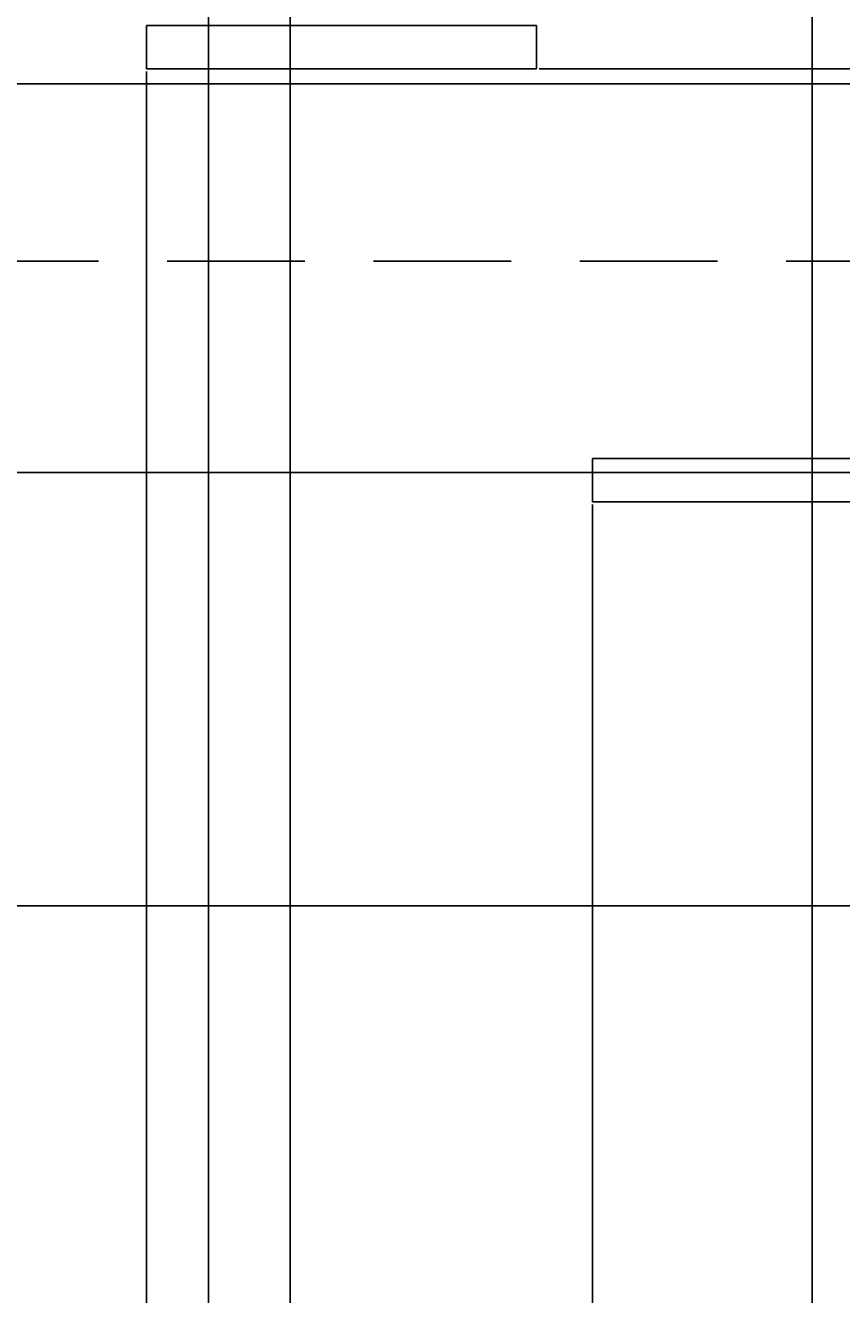
# Model space of a CAD drawing. Units: inches. Extents: x 2812 to 3051, y 1398 to 1659.
# Tile 31 of 65: x 2966 to 2985, y 1438 to 1468. Entities that reach past the tile are written whole.
import ezdxf

# ---------------------------------------------------------------- set-up
doc = ezdxf.new("R2010")
doc.units = ezdxf.units.IN
doc.linetypes.add('HIDDEN2', pattern=[4.7625, 3.175, -1.5875])
for name, color, linetype, lineweight in [('A-ANNO-DIMS', 2, 'Continuous', 18), ('S-CONC-HIDN', 8, 'HIDDEN2', 25), ('S-STEP', 3, 'Continuous', 25)]:
    doc.layers.add(name, color=color, linetype=linetype, lineweight=lineweight)
doc.styles.get("Standard").update_dxf_attribs({"font": 'arial.ttf'})
doc.dimstyles.get("Standard").update_dxf_attribs({"dimtxt": 0.18, "dimasz": 0.18, "dimexe": 0.18, "dimexo": 0.0625, "dimgap": 0.09, "dimtad": 0, "dimtih": 1, "dimtoh": 1, "dimdec": 4, "dimzin": 0, "dimdsep": 46, "dimtxsty": 'Standard', "dimcen": 0.09, "dimadec": 0, "dimazin": 0, "dimtfac": 1, "dimtdec": 4, "dimtofl": 0, "dimtmove": 0, "dimatfit": 3, "dimfxl": 1, "dimtolj": 1, "dimtzin": 0, "dimarcsym": 0})

# ---------------------------------------------------------------- blocks, each defined once
blk = doc.blocks.new('STEP-IRON-4')
for p, q in [((9, 1), (0, 1)), ((0, 1), (0, 0)), ((9, 0), (9, 1)), ((0, 0), (9, 0)), ((0, 0), (5.792, 0))]:
    blk.add_line(p, q)
blk = doc.blocks.new('STEP-IRON-5')
for p, q in [((9, 1), (0, 1)), ((0, 1), (0, 0)), ((9, 0), (9, 1)), ((0, 0), (9, 0))]:
    blk.add_line(p, q)
blk = doc.blocks.new('*D31')
at = {"layer": 'A-ANNO-DIMS', "color": 0, "lineweight": -2, "transparency": 16777216}
for p, q in [((2972.272, 1594.192), (2972.272, 1397.505)), ((2961.385, 1559.757), (2961.385, 1397.505)), ((2961.565, 1397.685), (2966.373, 1397.685)), ((2972.092, 1397.685), (2967.283, 1397.685))]:
    blk.add_line(p, q, dxfattribs=at)
at = {"layer": 'A-ANNO-DIMS', "color": 0, "transparency": 16777216}
for points in [[(2961.565, 1397.715), (2961.565, 1397.655), (2961.385, 1397.685)], [(2972.092, 1397.715), (2972.092, 1397.655), (2972.272, 1397.685)]]:
    blk.add_solid(points, dxfattribs=at)
at = {"layer": 'Defpoints', "color": 0, "transparency": 16777216}
for p in [(2972.272, 1594.254), (2961.385, 1559.82), (2972.272, 1397.685)]:
    blk.add_point(p, dxfattribs=at)
at = {"layer": 'A-ANNO-DIMS', "color": 0, "transparency": 16777216, "insert": (2966.828, 1397.685), "char_height": 0.18, "attachment_point": 5}
blk.add_mtext('\\A1;10.887', dxfattribs=at)
blk = doc.blocks.new('*D32')
at = {"layer": 'A-ANNO-DIMS', "color": 0, "lineweight": -2, "transparency": 16777216}
for p, q in [((2984.316, 1598.757), (2984.316, 1397.505)), ((2972.272, 1594.192), (2972.272, 1397.505)), ((2972.452, 1397.685), (2977.839, 1397.685)), ((2984.136, 1397.685), (2978.748, 1397.685))]:
    blk.add_line(p, q, dxfattribs=at)
at = {"layer": 'A-ANNO-DIMS', "color": 0, "transparency": 16777216}
for points in [[(2972.452, 1397.715), (2972.452, 1397.655), (2972.272, 1397.685)], [(2984.136, 1397.715), (2984.136, 1397.655), (2984.316, 1397.685)]]:
    blk.add_solid(points, dxfattribs=at)
at = {"layer": 'Defpoints', "color": 0, "transparency": 16777216}
for p in [(2984.316, 1598.82), (2972.272, 1594.254), (2984.316, 1397.685)]:
    blk.add_point(p, dxfattribs=at)
at = {"layer": 'A-ANNO-DIMS', "color": 0, "transparency": 16777216, "insert": (2978.294, 1397.685), "char_height": 0.18, "attachment_point": 5}
blk.add_mtext('\\A1;12.044', dxfattribs=at)
blk = doc.blocks.new('*D46')
at = {"layer": 'A-ANNO-DIMS', "color": 0, "lineweight": -2, "transparency": 16777216}
for p, q in [((2941.385, 1487.973), (2941.385, 1397.505)), ((2970.385, 1487.973), (2970.385, 1397.505)), ((2941.565, 1397.685), (2955.664, 1397.685)), ((2970.205, 1397.685), (2956.106, 1397.685))]:
    blk.add_line(p, q, dxfattribs=at)
at = {"layer": 'A-ANNO-DIMS', "color": 0, "transparency": 16777216}
for points in [[(2941.565, 1397.715), (2941.565, 1397.655), (2941.385, 1397.685)], [(2970.205, 1397.715), (2970.205, 1397.655), (2970.385, 1397.685)]]:
    blk.add_solid(points, dxfattribs=at)
at = {"layer": 'Defpoints', "color": 0, "transparency": 16777216}
for p in [(2941.385, 1488.035), (2970.385, 1488.035), (2970.385, 1397.685)]:
    blk.add_point(p, dxfattribs=at)
at = {"layer": 'A-ANNO-DIMS', "color": 0, "transparency": 16777216, "insert": (2955.885, 1397.685), "char_height": 0.18, "attachment_point": 5}
blk.add_mtext('\\A1;29', dxfattribs=at)
blk = doc.blocks.new('*D47')
at = {"layer": 'A-ANNO-DIMS', "color": 0, "lineweight": -2, "transparency": 16777216}
for p, q in [((2970.385, 1487.973), (2970.385, 1397.505)), ((3006.385, 1487.973), (3006.385, 1397.505)), ((2970.565, 1397.685), (2988.166, 1397.685)), ((3006.205, 1397.685), (2988.604, 1397.685))]:
    blk.add_line(p, q, dxfattribs=at)
at = {"layer": 'A-ANNO-DIMS', "color": 0, "transparency": 16777216}
for points in [[(2970.565, 1397.715), (2970.565, 1397.655), (2970.385, 1397.685)], [(3006.205, 1397.715), (3006.205, 1397.655), (3006.385, 1397.685)]]:
    blk.add_solid(points, dxfattribs=at)
at = {"layer": 'Defpoints', "color": 0, "transparency": 16777216}
for p in [(2970.385, 1488.035), (3006.385, 1488.035), (3006.385, 1397.685)]:
    blk.add_point(p, dxfattribs=at)
at = {"layer": 'A-ANNO-DIMS', "color": 0, "transparency": 16777216, "insert": (2988.385, 1397.685), "char_height": 0.18, "attachment_point": 5}
blk.add_mtext('\\A1;36', dxfattribs=at)
blk = doc.blocks.new('*D66')
at = {"layer": 'A-ANNO-DIMS', "color": 0, "lineweight": -2, "transparency": 16777216}
for p, q in [((2914.018, 1447.426), (3051.178, 1447.426)), ((3050.998, 1447.246), (3050.998, 1442.608)), ((3050.998, 1437.606), (3050.998, 1442.245)), ((2920.62, 1437.426), (3051.178, 1437.426))]:
    blk.add_line(p, q, dxfattribs=at)
at = {"layer": 'A-ANNO-DIMS', "color": 0, "transparency": 16777216}
for points in [[(3050.968, 1447.246), (3051.028, 1447.246), (3050.998, 1447.426)], [(3050.968, 1437.606), (3051.028, 1437.606), (3050.998, 1437.426)]]:
    blk.add_solid(points, dxfattribs=at)
at = {"layer": 'Defpoints', "color": 0, "transparency": 16777216}
for p in [(2913.955, 1447.426), (3050.998, 1447.426), (2920.558, 1437.426)]:
    blk.add_point(p, dxfattribs=at)
at = {"layer": 'A-ANNO-DIMS', "color": 0, "transparency": 16777216, "insert": (3050.998, 1442.426), "char_height": 0.18, "attachment_point": 5}
blk.add_mtext('\\A1;10', dxfattribs=at)
blk = doc.blocks.new('*D67')
at = {"layer": 'A-ANNO-DIMS', "color": 0, "lineweight": -2, "transparency": 16777216}
for p, q in [((2906.065, 1457.426), (3051.178, 1457.426)), ((3050.998, 1457.246), (3050.998, 1452.608)), ((3050.998, 1447.606), (3050.998, 1452.245)), ((2914.018, 1447.426), (3051.178, 1447.426))]:
    blk.add_line(p, q, dxfattribs=at)
at = {"layer": 'A-ANNO-DIMS', "color": 0, "transparency": 16777216}
for points in [[(3050.968, 1457.246), (3051.028, 1457.246), (3050.998, 1457.426)], [(3050.968, 1447.606), (3051.028, 1447.606), (3050.998, 1447.426)]]:
    blk.add_solid(points, dxfattribs=at)
at = {"layer": 'Defpoints', "color": 0, "transparency": 16777216}
for p in [(2906.002, 1457.426), (3050.998, 1457.426), (2913.955, 1447.426)]:
    blk.add_point(p, dxfattribs=at)
at = {"layer": 'A-ANNO-DIMS', "color": 0, "transparency": 16777216, "insert": (3050.998, 1452.426), "char_height": 0.18, "attachment_point": 5}
blk.add_mtext('\\A1;10', dxfattribs=at)
blk = doc.blocks.new('*D68')
at = {"layer": 'A-ANNO-DIMS', "color": 0, "lineweight": -2, "transparency": 16777216}
for p, q in [((2898.12, 1466.402), (3051.178, 1466.402)), ((3050.998, 1466.222), (3050.998, 1462.096)), ((3050.998, 1457.606), (3050.998, 1461.733)), ((2906.065, 1457.426), (3051.178, 1457.426))]:
    blk.add_line(p, q, dxfattribs=at)
at = {"layer": 'A-ANNO-DIMS', "color": 0, "transparency": 16777216}
for points in [[(3050.968, 1466.222), (3051.028, 1466.222), (3050.998, 1466.402)], [(3050.968, 1457.606), (3051.028, 1457.606), (3050.998, 1457.426)]]:
    blk.add_solid(points, dxfattribs=at)
at = {"layer": 'Defpoints', "color": 0, "transparency": 16777216}
for p in [(2898.058, 1466.402), (3050.998, 1466.402), (2906.002, 1457.426)]:
    blk.add_point(p, dxfattribs=at)
at = {"layer": 'A-ANNO-DIMS', "color": 0, "transparency": 16777216, "insert": (3050.998, 1461.914), "char_height": 0.18, "attachment_point": 5}
blk.add_mtext('\\A1;8.976', dxfattribs=at)
blk = doc.blocks.new('*D71')
at = {"layer": 'A-ANNO-DIMS', "color": 0, "lineweight": -2, "transparency": 16777216}
for p, q in [((2968.956, 1466.685), (2968.956, 1397.505)), ((2979.248, 1456.685), (2979.248, 1397.505)), ((2969.136, 1397.685), (2973.648, 1397.685)), ((2979.068, 1397.685), (2974.556, 1397.685))]:
    blk.add_line(p, q, dxfattribs=at)
at = {"layer": 'A-ANNO-DIMS', "color": 0, "transparency": 16777216}
for points in [[(2969.136, 1397.715), (2969.136, 1397.655), (2968.956, 1397.685)], [(2979.068, 1397.715), (2979.068, 1397.655), (2979.248, 1397.685)]]:
    blk.add_solid(points, dxfattribs=at)
at = {"layer": 'Defpoints', "color": 0, "transparency": 16777216}
for p in [(2968.956, 1466.747), (2979.248, 1456.747), (2979.248, 1397.685)]:
    blk.add_point(p, dxfattribs=at)
at = {"layer": 'A-ANNO-DIMS', "color": 0, "transparency": 16777216, "insert": (2974.102, 1397.685), "char_height": 0.18, "attachment_point": 5}
blk.add_mtext('\\A1;10.292', dxfattribs=at)
blk = doc.blocks.new('*D72')
at = {"layer": 'A-ANNO-DIMS', "color": 0, "lineweight": -2, "transparency": 16777216}
for p, q in [((2979.248, 1456.685), (2979.248, 1397.505)), ((2986.956, 1446.685), (2986.956, 1397.505)), ((2979.428, 1397.685), (2982.709, 1397.685)), ((2986.776, 1397.685), (2983.495, 1397.685))]:
    blk.add_line(p, q, dxfattribs=at)
at = {"layer": 'A-ANNO-DIMS', "color": 0, "transparency": 16777216}
for points in [[(2979.428, 1397.715), (2979.428, 1397.655), (2979.248, 1397.685)], [(2986.776, 1397.715), (2986.776, 1397.655), (2986.956, 1397.685)]]:
    blk.add_solid(points, dxfattribs=at)
at = {"layer": 'Defpoints', "color": 0, "transparency": 16777216}
for p in [(2979.248, 1456.747), (2986.956, 1446.747), (2986.956, 1397.685)]:
    blk.add_point(p, dxfattribs=at)
at = {"layer": 'A-ANNO-DIMS', "color": 0, "transparency": 16777216, "insert": (2983.102, 1397.685), "char_height": 0.18, "attachment_point": 5}
blk.add_mtext('\\A1;7.708', dxfattribs=at)
blk = doc.blocks.new('*D82')
at = {"layer": 'A-ANNO-DIMS', "color": 0, "lineweight": -2, "transparency": 16777216}
for p, q in [((2978.018, 1466.747), (3051.178, 1466.747)), ((3050.998, 1466.567), (3050.998, 1461.929)), ((3050.998, 1456.927), (3050.998, 1461.565)), ((2988.31, 1456.747), (3051.178, 1456.747))]:
    blk.add_line(p, q, dxfattribs=at)
at = {"layer": 'A-ANNO-DIMS', "color": 0, "transparency": 16777216}
for points in [[(3050.968, 1466.567), (3051.028, 1466.567), (3050.998, 1466.747)], [(3050.968, 1456.927), (3051.028, 1456.927), (3050.998, 1456.747)]]:
    blk.add_solid(points, dxfattribs=at)
at = {"layer": 'Defpoints', "color": 0, "transparency": 16777216}
for p in [(2977.956, 1466.747), (3050.998, 1466.747), (2988.248, 1456.747)]:
    blk.add_point(p, dxfattribs=at)
at = {"layer": 'A-ANNO-DIMS', "color": 0, "transparency": 16777216, "insert": (3050.998, 1461.747), "char_height": 0.18, "attachment_point": 5}
blk.add_mtext('\\A1;10', dxfattribs=at)

msp = doc.modelspace()

# ---------------------------------------------------------------- linework, layer by layer
at = {"layer": 'S-CONC-HIDN'}
msp.add_line((3029.7562, 1462.3026), (2835.3849, 1462.3026), dxfattribs=at)

# ---------------------------------------------------------------- block references
at = {"layer": 'S-STEP'}
for name, p in [('STEP-IRON-5', (2968.956, 1466.747)), ('STEP-IRON-4', (2979.248, 1456.747))]:
    msp.add_blockref(name, p, dxfattribs=at)

# ---------------------------------------------------------------- dimensions: what is measured, and where the dimension line sits
at = {"layer": 'A-ANNO-DIMS'}
for base, p1, p2, override, picture, middle in [((2984.3156, 1397.6854), (2972.2716, 1594.2541), (2984.3156, 1598.82), {"dimdec": 3, "dimlfac": 1, "dimrnd": 0, "dimzin": 0, "dimdsep": 46, "dimlunit": 2}, '*D32', (2978.2936, 1397.6854)), ((2972.2716, 1397.6854), (2961.3849, 1559.82), (2972.2716, 1594.2541), {"dimdec": 3, "dimlfac": 1, "dimrnd": 0, "dimzin": 0, "dimdsep": 46, "dimlunit": 2}, '*D31', (2966.8282, 1397.6854)), ((2970.3849, 1397.6854), (2941.3849, 1488.0354), (2970.3849, 1488.0354), {"dimdec": 0, "dimlfac": 1, "dimrnd": 0, "dimzin": 0, "dimdsep": 46, "dimlunit": 2}, '*D46', (2955.8849, 1397.6854)), ((3006.3849, 1397.6854), (2970.3849, 1488.0354), (3006.3849, 1488.0354), {"dimdec": 0, "dimlfac": 1, "dimrnd": 0, "dimzin": 0, "dimdsep": 46, "dimlunit": 2}, '*D47', (2988.3849, 1397.6854)), ((2979.2478, 1397.6854), (2968.9558, 1466.7474), (2979.2478, 1456.7474), {"dimdec": 3, "dimlfac": 1, "dimrnd": 0, "dimzin": 0, "dimdsep": 46, "dimlunit": 2}, '*D71', (2974.1018, 1397.6854)), ((2986.9558, 1397.6854), (2979.2478, 1456.7474), (2986.9558, 1446.7474), {"dimdec": 3, "dimlfac": 1, "dimrnd": 0, "dimzin": 0, "dimdsep": 46, "dimlunit": 2}, '*D72', (2983.1018, 1397.6854))]:
    dim = msp.add_linear_dim(base=base, p1=p1, p2=p2, dimstyle='Standard', override=override, dxfattribs=at)
    dim.commit()
    dim.dimension.update_dxf_attribs({"geometry": picture, "text_midpoint": middle})
for base, p1, p2, override, picture, middle in [((3050.998, 1466.7474), (2988.2478, 1456.7474), (2977.9558, 1466.7474), {"dimdec": 0, "dimlfac": 1, "dimrnd": 0, "dimzin": 0, "dimdsep": 46, "dimlunit": 2}, '*D82', (3050.998, 1461.7474)), ((3050.998, 1466.4024), (2906.0021, 1457.4265), (2898.0577, 1466.4024), {"dimdec": 3, "dimlfac": 1, "dimrnd": 0, "dimzin": 0, "dimdsep": 46, "dimlunit": 2}, '*D68', (3050.998, 1461.9144)), ((3050.998, 1457.4265), (2913.9551, 1447.4265), (2906.0021, 1457.4265), {"dimdec": 0, "dimlfac": 1, "dimrnd": 0, "dimzin": 0, "dimdsep": 46, "dimlunit": 2}, '*D67', (3050.998, 1452.4265)), ((3050.998, 1447.4265), (2920.5577, 1437.4265), (2913.9551, 1447.4265), {"dimdec": 0, "dimlfac": 1, "dimrnd": 0, "dimzin": 0, "dimdsep": 46, "dimlunit": 2}, '*D66', (3050.998, 1442.4265))]:
    dim = msp.add_linear_dim(base=base, p1=p1, p2=p2, angle=90, dimstyle='Standard', override=override, dxfattribs=at)
    dim.commit()
    dim.dimension.update_dxf_attribs({"geometry": picture, "text_midpoint": middle})

doc.saveas('drawing.dxf')
